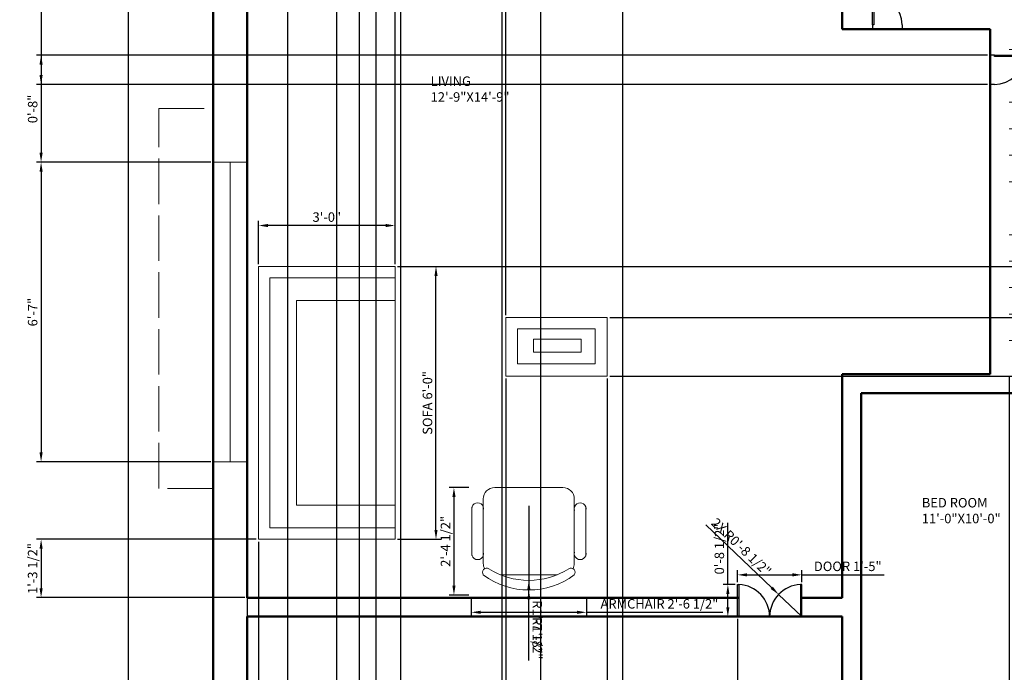
# Model space of a CAD drawing. Units: millimetres. Extents: x 3095 to 3505, y 1097 to 1734.
# Tile 2 of 5: x 3095 to 3355, y 1240 to 1412. Entities that reach past the tile are written whole.
import ezdxf

# ---------------------------------------------------------------- set-up
doc = ezdxf.new("R2010")
doc.units = ezdxf.units.MM
doc.linetypes.add('ACAD_ISO02W100', pattern=[15, 12, -3])
for name, color, linetype, lineweight, true_color in [('A-ANNO-DIMS', 32, 'Continuous', 18, 0xcd6928), ('A-AREA-IDEN', 152, 'Continuous', 18, 0x2776bb), ('A-FLOR-PATT', 241, 'Continuous', 13, 0xf7abae), ('A-FURN', 9, 'Continuous', 18, 0xafd9aa), ('A-GLAZ', 9, 'Continuous', 18, 0xd19cc7), ('A-ROOF-OVHD', 152, 'ACAD_ISO02W100', 13, 0x2776bb)]:
    doc.layers.add(name, color=color, linetype=linetype, lineweight=lineweight, true_color=true_color)
doc.layers.add('A-DOOR', color=4, linetype='Continuous', lineweight=25)
doc.layers.add('A-WALL', color=7, linetype='Continuous', lineweight=50)
doc.styles.get("Standard").update_dxf_attribs({"font": 'arial.ttf'})
doc.dimstyles.new('ISO-25', dxfattribs={"dimtxt": 2.5, "dimasz": 2.5, "dimexe": 1.25, "dimexo": 0.625, "dimtad": 1, "dimlunit": 3, "dimtxsty": 'Standard', "dimcen": 2.5, "dimadec": 0, "dimazin": 0, "dimtfac": 1, "dimtmove": 0, "dimatfit": 3, "dimfxl": 1, "dimarcsym": 0})

# ---------------------------------------------------------------- blocks, each defined once
blk = doc.blocks.new('CHAIR7')
for p, q in [((5.12, 15.04), (17.88, 15.04)), ((20, 12), (3, 12)), ((0, 9), (0, -9)), ((23, -7.44), (23, 7.44)), ((3, -12), (20, -12)), ((5.12, -15), (17.88, -15))]:
    blk.add_line(p, q)
for centre, radius, start, end in [((5.56, 13.54), 1.56, 73.7398, 286.2602), ((17.44, 13.54), 1.56, 253.7398, 106.2602), ((3, 9), 3, 90, 180), ((20, 9), 3, 62.4156, 90), ((22.34, 11.12), 1.1, 53.3099, 212.0274), ((4.82, 0), 19.64, 327.5758, 32.4242), ((7, 0), 20, 323.1301, 36.8699), ((3, -9), 3, 180, 270), ((5.56, -13.5), 1.56, 73.7398, 286.2602), ((17.44, -13.5), 1.56, 253.7398, 106.2602), ((20, -9), 3, 270, 297.5844), ((22.34, -11.12), 1.1, 147.9726, 306.6901)]:
    blk.add_arc(centre, radius, start, end)
blk = doc.blocks.new('SOFA2')
for p, q in [((-36, 0), (-36, -36)), ((36, 0), (-36, 0)), ((36, -36), (36, 0)), ((-33, -36), (-33, -3)), ((-33, -3), (33, -3)), ((33, -3), (33, -36)), ((-27, -36), (-27, -10)), ((-27, -10), (27, -10)), ((27, -10), (27, -36)), ((-36, -36), (36, -36))]:
    blk.add_line(p, q)
blk = doc.blocks.new('*U6')
for p, q in [((0, 0), (0, -6)), ((40, 0), (40, -6))]:
    blk.add_line(p, q)
blk.add_lwpolyline([(0, 0), (0, 40), (1.75, 40), (1.75, 0)], close=True)
blk.add_arc((0, 0), 40, 0, 90)
blk = doc.blocks.new('*U8')
for p, q in [((0, 0), (0, -6)), ((40, 0), (40, -6))]:
    blk.add_line(p, q)
blk.add_lwpolyline([(0, 0), (0, 40), (1.75, 40), (1.75, 0)], close=True)
blk.add_arc((0, 0), 40, 0, 90)
blk = doc.blocks.new('DR-69P')
for points in [[(1.5, 0), (0, 0), (0, 34.5), (1.5, 34.5)], [(67.5, 0), (69, 0), (69, 34.5), (67.5, 34.5)]]:
    blk.add_lwpolyline(points, close=True)
for centre, start, end in [((0, 0), 0, 87.5104), ((69, 0), 92.4896, 180)]:
    blk.add_arc(centre, 34.5, start, end)
blk = doc.blocks.new('*D11')
at = {"layer": 'A-ANNO-DIMS', "color": 0, "lineweight": -2, "transparency": 16777216}
for p, q in [((3145.24, 1677.32), (3122.17, 1677.32)), ((3123.42, 1674.82), (3123.42, 1175.82)), ((3145.24, 1173.32), (3122.17, 1173.32))]:
    blk.add_line(p, q, dxfattribs=at)
at = {"layer": 'A-ANNO-DIMS', "color": 0, "lineweight": 5, "transparency": 16777216}
for points in [[(3123, 1674.82), (3123.84, 1674.82), (3123.42, 1677.32)], [(3123, 1175.82), (3123.84, 1175.82), (3123.42, 1173.32)]]:
    blk.add_solid(points, dxfattribs=at)
at = {"layer": 'Defpoints', "color": 0, "lineweight": 5, "transparency": 16777216}
for p in [(3145.86, 1677.32), (3123.42, 1173.32), (3145.86, 1173.32)]:
    blk.add_point(p, dxfattribs=at)
at = {"layer": 'A-ANNO-DIMS', "color": 0, "transparency": 16777216, "insert": (3121.54, 1425.32), "char_height": 2.5, "attachment_point": 5, "rotation": 90}
blk.add_mtext("42'", dxfattribs=at)
blk = doc.blocks.new('*D24')
at = {"layer": 'A-ANNO-DIMS', "color": 0, "lineweight": -2, "transparency": 16777216}
for p, q in [((3213.96, 1259.39), (3213.96, 1254.21)), ((3244.38, 1259.39), (3244.38, 1254.21)), ((3216.46, 1255.46), (3241.88, 1255.46)), ((3244.38, 1255.46), (3280.34, 1255.46))]:
    blk.add_line(p, q, dxfattribs=at)
at = {"layer": 'A-ANNO-DIMS', "color": 0, "lineweight": 5, "transparency": 16777216}
for points in [[(3216.46, 1255.87), (3216.46, 1255.04), (3213.96, 1255.46)], [(3241.88, 1255.87), (3241.88, 1255.04), (3244.38, 1255.46)]]:
    blk.add_solid(points, dxfattribs=at)
at = {"layer": 'Defpoints', "color": 0, "lineweight": 5, "transparency": 16777216}
for p in [(3213.96, 1260.02), (3244.38, 1260.02), (3244.38, 1255.46)]:
    blk.add_point(p, dxfattribs=at)
at = {"layer": 'A-ANNO-DIMS', "color": 0, "transparency": 16777216, "insert": (3263.61, 1257.37), "char_height": 2.5, "attachment_point": 5}
blk.add_mtext('ARMCHAIR 2\'-6 1/2"', dxfattribs=at)
blk = doc.blocks.new('*D25')
at = {"layer": 'A-ANNO-DIMS', "color": 0, "lineweight": -2, "transparency": 16777216}
for p, q in [((3213.34, 1288.35), (3208.15, 1288.35)), ((3209.4, 1285.85), (3209.4, 1262.52)), ((3213.34, 1260.02), (3208.15, 1260.02))]:
    blk.add_line(p, q, dxfattribs=at)
at = {"layer": 'A-ANNO-DIMS', "color": 0, "lineweight": 5, "transparency": 16777216}
for points in [[(3208.98, 1285.85), (3209.82, 1285.85), (3209.4, 1288.35)], [(3208.98, 1262.52), (3209.82, 1262.52), (3209.4, 1260.02)]]:
    blk.add_solid(points, dxfattribs=at)
at = {"layer": 'Defpoints', "color": 0, "lineweight": 5, "transparency": 16777216}
for p in [(3213.96, 1288.35), (3209.4, 1260.02), (3213.96, 1260.02)]:
    blk.add_point(p, dxfattribs=at)
at = {"layer": 'A-ANNO-DIMS', "color": 0, "transparency": 16777216, "insert": (3207.48, 1274.18), "char_height": 2.5, "attachment_point": 5, "rotation": 90}
blk.add_mtext('2\'-4 1/2"', dxfattribs=at)
blk = doc.blocks.new('*D26')
at = {"layer": 'A-ANNO-DIMS', "color": 0, "lineweight": -2, "transparency": 16777216}
for p, q in [((3194.49, 1346.71), (3205.91, 1346.71)), ((3204.66, 1277.21), (3204.66, 1344.21)), ((3194.49, 1274.71), (3205.91, 1274.71))]:
    blk.add_line(p, q, dxfattribs=at)
at = {"layer": 'A-ANNO-DIMS', "color": 0, "lineweight": 5, "transparency": 16777216}
for points in [[(3204.25, 1344.21), (3205.08, 1344.21), (3204.66, 1346.71)], [(3204.25, 1277.21), (3205.08, 1277.21), (3204.66, 1274.71)]]:
    blk.add_solid(points, dxfattribs=at)
at = {"layer": 'Defpoints', "color": 0, "lineweight": 5, "transparency": 16777216}
for p in [(3193.86, 1346.71), (3204.66, 1346.71), (3193.86, 1274.71)]:
    blk.add_point(p, dxfattribs=at)
at = {"layer": 'A-ANNO-DIMS', "color": 0, "transparency": 16777216, "insert": (3202.74, 1310.71), "char_height": 2.5, "attachment_point": 5, "rotation": 90}
blk.add_mtext('SOFA 6\'-0"', dxfattribs=at)
blk = doc.blocks.new('*D27')
at = {"layer": 'A-ANNO-DIMS', "color": 0, "lineweight": -2, "transparency": 16777216}
for p, q in [((3157.86, 1347.34), (3157.86, 1358.76)), ((3193.86, 1347.34), (3193.86, 1358.76)), ((3191.36, 1357.51), (3160.36, 1357.51))]:
    blk.add_line(p, q, dxfattribs=at)
at = {"layer": 'A-ANNO-DIMS', "color": 0, "lineweight": 5, "transparency": 16777216}
for points in [[(3160.36, 1357.93), (3160.36, 1357.09), (3157.86, 1357.51)], [(3191.36, 1357.93), (3191.36, 1357.09), (3193.86, 1357.51)]]:
    blk.add_solid(points, dxfattribs=at)
at = {"layer": 'Defpoints', "color": 0, "lineweight": 5, "transparency": 16777216}
for p in [(3157.86, 1357.51), (3157.86, 1346.71), (3193.86, 1346.71)]:
    blk.add_point(p, dxfattribs=at)
at = {"layer": 'A-ANNO-DIMS', "color": 0, "transparency": 16777216, "insert": (3175.86, 1359.41), "char_height": 2.5, "attachment_point": 5}
blk.add_mtext('3\'-0"', dxfattribs=at)
blk = doc.blocks.new('*D28')
at = {"layer": 'A-ANNO-DIMS', "color": 0, "lineweight": -2, "transparency": 16777216}
for p, q in [((3284.21, 1263.42), (3284.21, 1266.59)), ((3286.71, 1265.34), (3298.68, 1265.34)), ((3301.18, 1263.42), (3301.18, 1266.59)), ((3301.18, 1265.34), (3322.9, 1265.34))]:
    blk.add_line(p, q, dxfattribs=at)
at = {"layer": 'A-ANNO-DIMS', "color": 0, "lineweight": 5, "transparency": 16777216}
for points in [[(3286.71, 1265.76), (3286.71, 1264.92), (3284.21, 1265.34)], [(3298.68, 1265.76), (3298.68, 1264.92), (3301.18, 1265.34)]]:
    blk.add_solid(points, dxfattribs=at)
at = {"layer": 'Defpoints', "color": 0, "lineweight": 5, "transparency": 16777216}
for p in [(3301.18, 1265.34), (3284.21, 1262.8), (3301.18, 1262.8)]:
    blk.add_point(p, dxfattribs=at)
at = {"layer": 'A-ANNO-DIMS', "color": 0, "transparency": 16777216, "insert": (3313.29, 1267.26), "char_height": 2.5, "attachment_point": 5}
blk.add_mtext('DOOR 1\'-5"', dxfattribs=at)
blk = doc.blocks.new('*D29')
at = {"layer": 'A-ANNO-DIMS', "color": 0, "lineweight": -2, "transparency": 16777216}
for p, q in [((3281.66, 1262.8), (3281.66, 1279.02)), ((3283.58, 1262.8), (3280.41, 1262.8)), ((3281.66, 1256.81), (3281.66, 1260.3)), ((3283.58, 1254.31), (3280.41, 1254.31))]:
    blk.add_line(p, q, dxfattribs=at)
at = {"layer": 'A-ANNO-DIMS', "color": 0, "lineweight": 5, "transparency": 16777216}
for points in [[(3281.24, 1260.3), (3282.08, 1260.3), (3281.66, 1262.8)], [(3281.24, 1256.81), (3282.08, 1256.81), (3281.66, 1254.31)]]:
    blk.add_solid(points, dxfattribs=at)
at = {"layer": 'Defpoints', "color": 0, "lineweight": 5, "transparency": 16777216}
for p in [(3281.66, 1262.8), (3284.21, 1262.8), (3284.21, 1254.31)]:
    blk.add_point(p, dxfattribs=at)
at = {"layer": 'A-ANNO-DIMS', "color": 0, "transparency": 16777216, "insert": (3279.74, 1272.16), "char_height": 2.5, "attachment_point": 5, "rotation": 90}
blk.add_mtext('0\'-8 1/2"', dxfattribs=at)
blk = doc.blocks.new('*D36')
at = {"layer": 'A-ANNO-DIMS', "color": 0, "lineweight": -2, "transparency": 16777216}
for p, q in [((3145.24, 1477.6), (3099.22, 1477.6)), ((3100.47, 1475.1), (3100.47, 1376.7)), ((3145.24, 1374.2), (3099.22, 1374.2))]:
    blk.add_line(p, q, dxfattribs=at)
at = {"layer": 'A-ANNO-DIMS', "color": 0, "lineweight": 5, "transparency": 16777216}
for points in [[(3100.06, 1475.1), (3100.89, 1475.1), (3100.47, 1477.6)], [(3100.06, 1376.7), (3100.89, 1376.7), (3100.47, 1374.2)]]:
    blk.add_solid(points, dxfattribs=at)
at = {"layer": 'Defpoints', "color": 0, "lineweight": 5, "transparency": 16777216}
for p in [(3145.86, 1477.6), (3100.47, 1374.2), (3145.86, 1374.2)]:
    blk.add_point(p, dxfattribs=at)
at = {"layer": 'A-ANNO-DIMS', "color": 0, "transparency": 16777216, "insert": (3098.56, 1425.9), "char_height": 2.5, "attachment_point": 5, "rotation": 90}
blk.add_mtext('8\'-7 1/2"', dxfattribs=at)
blk = doc.blocks.new('*D37')
at = {"layer": 'A-ANNO-DIMS', "color": 0, "lineweight": -2, "transparency": 16777216}
for p, q in [((3145.24, 1374.2), (3099.22, 1374.2)), ((3100.47, 1371.7), (3100.47, 1297.63)), ((3145.24, 1295.13), (3099.22, 1295.13))]:
    blk.add_line(p, q, dxfattribs=at)
at = {"layer": 'A-ANNO-DIMS', "color": 0, "lineweight": 5, "transparency": 16777216}
for points in [[(3100.06, 1371.7), (3100.89, 1371.7), (3100.47, 1374.2)], [(3100.06, 1297.63), (3100.89, 1297.63), (3100.47, 1295.13)]]:
    blk.add_solid(points, dxfattribs=at)
at = {"layer": 'Defpoints', "color": 0, "lineweight": 5, "transparency": 16777216}
for p in [(3145.86, 1374.2), (3100.47, 1295.13), (3145.86, 1295.13)]:
    blk.add_point(p, dxfattribs=at)
at = {"layer": 'A-ANNO-DIMS', "color": 0, "transparency": 16777216, "insert": (3098.57, 1334.66), "char_height": 2.5, "attachment_point": 5, "rotation": 90}
blk.add_mtext('6\'-7"', dxfattribs=at)
blk = doc.blocks.new('*D49')
at = {"layer": 'A-ANNO-DIMS', "color": 0, "lineweight": -2, "transparency": 16777216}
for p, q in [((3154.86, 1588.17), (3154.86, 1134.75)), ((3188.81, 1588.17), (3188.81, 1134.75)), ((3157.36, 1136), (3186.31, 1136))]:
    blk.add_line(p, q, dxfattribs=at)
at = {"layer": 'A-ANNO-DIMS', "color": 0, "lineweight": 5, "transparency": 16777216}
for points in [[(3157.36, 1136.41), (3157.36, 1135.58), (3154.86, 1136)], [(3186.31, 1136.41), (3186.31, 1135.58), (3188.81, 1136)]]:
    blk.add_solid(points, dxfattribs=at)
at = {"layer": 'Defpoints', "color": 0, "lineweight": 5, "transparency": 16777216}
for p in [(3154.86, 1588.8), (3188.81, 1588.8), (3188.81, 1136)]:
    blk.add_point(p, dxfattribs=at)
at = {"layer": 'A-ANNO-DIMS', "color": 0, "transparency": 16777216, "insert": (3171.84, 1137.9), "char_height": 2.5, "attachment_point": 5}
blk.add_mtext('2\'-10"', dxfattribs=at)
blk = doc.blocks.new('*D50')
at = {"layer": 'A-ANNO-DIMS', "color": 0, "lineweight": -2, "transparency": 16777216}
for p, q in [((3222, 1588.17), (3222, 1134.75)), ((3253.86, 1588.17), (3253.86, 1134.75)), ((3224.5, 1136), (3251.36, 1136))]:
    blk.add_line(p, q, dxfattribs=at)
at = {"layer": 'A-ANNO-DIMS', "color": 0, "lineweight": 5, "transparency": 16777216}
for points in [[(3224.5, 1136.41), (3224.5, 1135.58), (3222, 1136)], [(3251.36, 1136.41), (3251.36, 1135.58), (3253.86, 1136)]]:
    blk.add_solid(points, dxfattribs=at)
at = {"layer": 'Defpoints', "color": 0, "lineweight": 5, "transparency": 16777216}
for p in [(3222, 1588.8), (3253.86, 1588.8), (3253.86, 1136)]:
    blk.add_point(p, dxfattribs=at)
at = {"layer": 'A-ANNO-DIMS', "color": 0, "transparency": 16777216, "insert": (3237.93, 1137.9), "char_height": 2.5, "attachment_point": 5}
blk.add_mtext('2\'-8"', dxfattribs=at)
blk = doc.blocks.new('*D52')
at = {"layer": 'A-ANNO-DIMS', "color": 0, "lineweight": -2, "transparency": 16777216}
for p, q in [((3178.42, 1456.63), (3178.42, 1134.75)), ((3232.26, 1456.63), (3232.26, 1134.75)), ((3180.92, 1136), (3229.76, 1136))]:
    blk.add_line(p, q, dxfattribs=at)
at = {"layer": 'A-ANNO-DIMS', "color": 0, "lineweight": 5, "transparency": 16777216}
for points in [[(3180.92, 1136.41), (3180.92, 1135.58), (3178.42, 1136)], [(3229.76, 1136.41), (3229.76, 1135.58), (3232.26, 1136)]]:
    blk.add_solid(points, dxfattribs=at)
at = {"layer": 'Defpoints', "color": 0, "lineweight": 5, "transparency": 16777216}
for p in [(3178.42, 1457.25), (3232.26, 1457.25), (3232.26, 1136)]:
    blk.add_point(p, dxfattribs=at)
at = {"layer": 'A-ANNO-DIMS', "color": 0, "transparency": 16777216, "insert": (3205.34, 1137.9), "char_height": 2.5, "attachment_point": 5}
blk.add_mtext('4\'-6"', dxfattribs=at)
blk = doc.blocks.new('*D57')
at = {"layer": 'A-ANNO-DIMS', "color": 0, "lineweight": -2, "transparency": 16777216}
for p, q in [((3165.47, 1598.31), (3165.47, 1134.75)), ((3184.42, 1598.31), (3184.42, 1134.75)), ((3167.97, 1136), (3181.92, 1136))]:
    blk.add_line(p, q, dxfattribs=at)
at = {"layer": 'A-ANNO-DIMS', "color": 0, "lineweight": 5, "transparency": 16777216}
for points in [[(3167.97, 1136.41), (3167.97, 1135.58), (3165.47, 1136)], [(3181.92, 1136.41), (3181.92, 1135.58), (3184.42, 1136)]]:
    blk.add_solid(points, dxfattribs=at)
at = {"layer": 'Defpoints', "color": 0, "lineweight": 5, "transparency": 16777216}
for p in [(3165.47, 1598.93), (3184.42, 1598.93), (3184.42, 1136)]:
    blk.add_point(p, dxfattribs=at)
at = {"layer": 'A-ANNO-DIMS', "color": 0, "transparency": 16777216, "insert": (3174.95, 1137.88), "char_height": 2.5, "attachment_point": 5}
blk.add_mtext('1\'-7"', dxfattribs=at)
blk = doc.blocks.new('*D62')
at = {"layer": 'A-ANNO-DIMS', "color": 0, "lineweight": -2, "transparency": 16777216}
for p, q in [((3350.19, 1402.48), (3099.22, 1402.48)), ((3100.47, 1399.98), (3100.47, 1397.22)), ((3350.19, 1394.72), (3099.22, 1394.72)), ((3100.47, 1394.72), (3100.47, 1384.32))]:
    blk.add_line(p, q, dxfattribs=at)
at = {"layer": 'A-ANNO-DIMS', "color": 0, "lineweight": 5, "transparency": 16777216}
for points in [[(3100.06, 1399.98), (3100.89, 1399.98), (3100.47, 1402.48)], [(3100.06, 1397.22), (3100.89, 1397.22), (3100.47, 1394.72)]]:
    blk.add_solid(points, dxfattribs=at)
at = {"layer": 'Defpoints', "color": 0, "lineweight": 5, "transparency": 16777216}
for p in [(3350.82, 1402.48), (3100.47, 1394.72), (3350.82, 1394.72)]:
    blk.add_point(p, dxfattribs=at)
at = {"layer": 'A-ANNO-DIMS', "color": 0, "transparency": 16777216, "insert": (3098.57, 1388.27), "char_height": 2.5, "attachment_point": 5, "rotation": 90}
blk.add_mtext('0\'-8"', dxfattribs=at)
blk = doc.blocks.new('*D64')
at = {"layer": 'A-ANNO-DIMS', "color": 0, "lineweight": -2, "transparency": 16777216}
for p, q in [((3355.86, 1317.69), (3355.86, 1134.75)), ((3356.76, 1312.81), (3356.76, 1134.75)), ((3353.36, 1136), (3342.97, 1136)), ((3356.76, 1136), (3355.86, 1136)), ((3359.26, 1136), (3361.76, 1136))]:
    blk.add_line(p, q, dxfattribs=at)
at = {"layer": 'A-ANNO-DIMS', "color": 0, "lineweight": 5, "transparency": 16777216}
for points in [[(3353.36, 1136.41), (3353.36, 1135.58), (3355.86, 1136)], [(3359.26, 1136.41), (3359.26, 1135.58), (3356.76, 1136)]]:
    blk.add_solid(points, dxfattribs=at)
at = {"layer": 'Defpoints', "color": 0, "lineweight": 5, "transparency": 16777216}
for p in [(3355.86, 1318.32), (3356.76, 1313.43), (3355.86, 1136)]:
    blk.add_point(p, dxfattribs=at)
at = {"layer": 'A-ANNO-DIMS', "color": 0, "transparency": 16777216, "insert": (3346.91, 1137.9), "char_height": 2.5, "attachment_point": 5}
blk.add_mtext('0\'-1"', dxfattribs=at)
blk = doc.blocks.new('*D65')
at = {"layer": 'A-ANNO-DIMS', "color": 0, "lineweight": -2, "transparency": 16777216}
for p, q in [((3178.42, 1456.63), (3178.42, 1134.75)), ((3154.86, 1439.69), (3154.86, 1134.75)), ((3175.92, 1136), (3157.36, 1136))]:
    blk.add_line(p, q, dxfattribs=at)
at = {"layer": 'A-ANNO-DIMS', "color": 0, "lineweight": 5, "transparency": 16777216}
for points in [[(3157.36, 1136.41), (3157.36, 1135.58), (3154.86, 1136)], [(3175.92, 1136.41), (3175.92, 1135.58), (3178.42, 1136)]]:
    blk.add_solid(points, dxfattribs=at)
at = {"layer": 'Defpoints', "color": 0, "lineweight": 5, "transparency": 16777216}
for p in [(3178.42, 1457.25), (3154.86, 1440.32), (3154.86, 1136)]:
    blk.add_point(p, dxfattribs=at)
at = {"layer": 'A-ANNO-DIMS', "color": 0, "transparency": 16777216, "insert": (3166.64, 1137.91), "char_height": 2.5, "attachment_point": 5}
blk.add_mtext('1\'-11 1/2"', dxfattribs=at)
blk = doc.blocks.new('*D67')
at = {"layer": 'A-ANNO-DIMS', "color": 0, "lineweight": -2, "transparency": 16777216}
for p, q in [((3154.86, 1253.69), (3154.86, 1134.75)), ((3284.21, 1253.69), (3284.21, 1134.75)), ((3281.71, 1136), (3157.36, 1136))]:
    blk.add_line(p, q, dxfattribs=at)
at = {"layer": 'A-ANNO-DIMS', "color": 0, "lineweight": 5, "transparency": 16777216}
for points in [[(3157.36, 1136.41), (3157.36, 1135.58), (3154.86, 1136)], [(3281.71, 1136.41), (3281.71, 1135.58), (3284.21, 1136)]]:
    blk.add_solid(points, dxfattribs=at)
at = {"layer": 'Defpoints', "color": 0, "lineweight": 5, "transparency": 16777216}
for p in [(3154.86, 1254.32), (3284.21, 1254.31), (3154.86, 1136)]:
    blk.add_point(p, dxfattribs=at)
at = {"layer": 'A-ANNO-DIMS', "color": 0, "transparency": 16777216, "insert": (3219.53, 1137.91), "char_height": 2.5, "attachment_point": 5}
blk.add_mtext('10\'-9 1/2"', dxfattribs=at)
blk = doc.blocks.new('*D68')
at = {"layer": 'A-ANNO-DIMS', "color": 0, "lineweight": -2, "transparency": 16777216}
for p, q in [((3223.06, 1317.18), (3223.06, 1134.75)), ((3249.85, 1317.18), (3249.85, 1134.75)), ((3225.56, 1136), (3247.35, 1136))]:
    blk.add_line(p, q, dxfattribs=at)
at = {"layer": 'A-ANNO-DIMS', "color": 0, "lineweight": 5, "transparency": 16777216}
for points in [[(3225.56, 1136.41), (3225.56, 1135.58), (3223.06, 1136)], [(3247.35, 1136.41), (3247.35, 1135.58), (3249.85, 1136)]]:
    blk.add_solid(points, dxfattribs=at)
at = {"layer": 'Defpoints', "color": 0, "lineweight": 5, "transparency": 16777216}
for p in [(3223.06, 1317.8), (3249.85, 1317.8), (3249.85, 1136)]:
    blk.add_point(p, dxfattribs=at)
at = {"layer": 'A-ANNO-DIMS', "color": 0, "transparency": 16777216, "insert": (3236.46, 1137.9), "char_height": 2.5, "attachment_point": 5}
blk.add_mtext('2\'-3"', dxfattribs=at)
blk = doc.blocks.new('*D69')
at = {"layer": 'A-ANNO-DIMS', "color": 0, "lineweight": -2, "transparency": 16777216}
for p, q in [((3250.48, 1333.27), (3504.29, 1333.27)), ((3503.04, 1330.77), (3503.04, 1320.3)), ((3250.48, 1317.8), (3504.29, 1317.8))]:
    blk.add_line(p, q, dxfattribs=at)
at = {"layer": 'A-ANNO-DIMS', "color": 0, "lineweight": 5, "transparency": 16777216}
for points in [[(3502.63, 1330.77), (3503.46, 1330.77), (3503.04, 1333.27)], [(3502.63, 1320.3), (3503.46, 1320.3), (3503.04, 1317.8)]]:
    blk.add_solid(points, dxfattribs=at)
at = {"layer": 'Defpoints', "color": 0, "lineweight": 5, "transparency": 16777216}
for p in [(3249.85, 1333.27), (3249.85, 1317.8), (3503.04, 1317.8)]:
    blk.add_point(p, dxfattribs=at)
at = {"layer": 'A-ANNO-DIMS', "color": 0, "transparency": 16777216, "insert": (3501.12, 1325.54), "char_height": 2.5, "attachment_point": 5, "rotation": 90}
blk.add_mtext('1\'-3 1/2"', dxfattribs=at)
blk = doc.blocks.new('*D70')
at = {"layer": 'A-ANNO-DIMS', "color": 0, "lineweight": -2, "transparency": 16777216}
for p, q in [((3165.47, 1598.31), (3165.47, 1134.75)), ((3154.86, 1588.17), (3154.86, 1134.75)), ((3157.36, 1136), (3162.97, 1136)), ((3165.47, 1136), (3183.64, 1136))]:
    blk.add_line(p, q, dxfattribs=at)
at = {"layer": 'A-ANNO-DIMS', "color": 0, "lineweight": 5, "transparency": 16777216}
for points in [[(3157.36, 1136.41), (3157.36, 1135.58), (3154.86, 1136)], [(3162.97, 1136.41), (3162.97, 1135.58), (3165.47, 1136)]]:
    blk.add_solid(points, dxfattribs=at)
at = {"layer": 'Defpoints', "color": 0, "lineweight": 5, "transparency": 16777216}
for p in [(3165.47, 1598.93), (3154.86, 1588.8), (3165.47, 1136)]:
    blk.add_point(p, dxfattribs=at)
at = {"layer": 'A-ANNO-DIMS', "color": 0, "transparency": 16777216, "insert": (3175.81, 1137.91), "char_height": 2.5, "attachment_point": 5}
blk.add_mtext('0\'-10 1/2"', dxfattribs=at)
blk = doc.blocks.new('*D72')
at = {"layer": 'A-ANNO-DIMS', "color": 0, "lineweight": -2, "transparency": 16777216}
for p, q in [((3195.33, 1651.97), (3195.33, 1134.75)), ((3188.81, 1649.1), (3188.81, 1134.75)), ((3188.81, 1136), (3172.59, 1136)), ((3192.83, 1136), (3191.31, 1136))]:
    blk.add_line(p, q, dxfattribs=at)
at = {"layer": 'A-ANNO-DIMS', "color": 0, "lineweight": 5, "transparency": 16777216}
for points in [[(3191.31, 1136.41), (3191.31, 1135.58), (3188.81, 1136)], [(3192.83, 1136.41), (3192.83, 1135.58), (3195.33, 1136)]]:
    blk.add_solid(points, dxfattribs=at)
at = {"layer": 'Defpoints', "color": 0, "lineweight": 5, "transparency": 16777216}
for p in [(3195.33, 1652.6), (3188.81, 1649.73), (3188.81, 1136)]:
    blk.add_point(p, dxfattribs=at)
at = {"layer": 'A-ANNO-DIMS', "color": 0, "transparency": 16777216, "insert": (3179.45, 1137.91), "char_height": 2.5, "attachment_point": 5}
blk.add_mtext('0\'-6 1/2"', dxfattribs=at)
blk = doc.blocks.new('*D74')
at = {"layer": 'A-ANNO-DIMS', "color": 0, "lineweight": -2, "transparency": 16777216}
for p, q in [((3157.86, 1274.09), (3157.86, 1134.75)), ((3154.86, 1258.69), (3154.86, 1134.75)), ((3152.36, 1136), (3141.97, 1136)), ((3157.86, 1136), (3154.86, 1136)), ((3160.36, 1136), (3162.86, 1136))]:
    blk.add_line(p, q, dxfattribs=at)
at = {"layer": 'A-ANNO-DIMS', "color": 0, "lineweight": 5, "transparency": 16777216}
for points in [[(3152.36, 1136.41), (3152.36, 1135.58), (3154.86, 1136)], [(3160.36, 1136.41), (3160.36, 1135.58), (3157.86, 1136)]]:
    blk.add_solid(points, dxfattribs=at)
at = {"layer": 'Defpoints', "color": 0, "lineweight": 5, "transparency": 16777216}
for p in [(3157.86, 1274.71), (3154.86, 1259.32), (3154.86, 1136)]:
    blk.add_point(p, dxfattribs=at)
at = {"layer": 'A-ANNO-DIMS', "color": 0, "transparency": 16777216, "insert": (3145.91, 1137.9), "char_height": 2.5, "attachment_point": 5}
blk.add_mtext('0\'-3"', dxfattribs=at)
blk = doc.blocks.new('*D75')
at = {"layer": 'A-ANNO-DIMS', "color": 0, "lineweight": -2, "transparency": 16777216}
for p, q in [((3157.24, 1274.71), (3099.22, 1274.71)), ((3100.47, 1272.21), (3100.47, 1261.82)), ((3154.24, 1259.32), (3099.22, 1259.32))]:
    blk.add_line(p, q, dxfattribs=at)
at = {"layer": 'A-ANNO-DIMS', "color": 0, "lineweight": 5, "transparency": 16777216}
for points in [[(3100.06, 1272.21), (3100.89, 1272.21), (3100.47, 1274.71)], [(3100.06, 1261.82), (3100.89, 1261.82), (3100.47, 1259.32)]]:
    blk.add_solid(points, dxfattribs=at)
at = {"layer": 'Defpoints', "color": 0, "lineweight": 5, "transparency": 16777216}
for p in [(3157.86, 1274.71), (3100.47, 1259.32), (3154.86, 1259.32)]:
    blk.add_point(p, dxfattribs=at)
at = {"layer": 'A-ANNO-DIMS', "color": 0, "transparency": 16777216, "insert": (3098.56, 1267.01), "char_height": 2.5, "attachment_point": 5, "rotation": 90}
blk.add_mtext('1\'-3 1/2"', dxfattribs=at)
blk = doc.blocks.new('*D76')
at = {"layer": 'A-ANNO-DIMS', "color": 0, "lineweight": -2, "transparency": 16777216}
for p, q in [((3193.86, 1347.34), (3193.86, 1729.27)), ((3196.36, 1728.02), (3220.56, 1728.02)), ((3223.06, 1333.89), (3223.06, 1729.27))]:
    blk.add_line(p, q, dxfattribs=at)
at = {"layer": 'A-ANNO-DIMS', "color": 0, "lineweight": 5, "transparency": 16777216}
for points in [[(3196.36, 1728.43), (3196.36, 1727.6), (3193.86, 1728.02)], [(3220.56, 1728.43), (3220.56, 1727.6), (3223.06, 1728.02)]]:
    blk.add_solid(points, dxfattribs=at)
at = {"layer": 'Defpoints', "color": 0, "lineweight": 5, "transparency": 16777216}
for p in [(3223.06, 1728.02), (3193.86, 1346.71), (3223.06, 1333.27)]:
    blk.add_point(p, dxfattribs=at)
at = {"layer": 'A-ANNO-DIMS', "color": 0, "transparency": 16777216, "insert": (3208.46, 1729.92), "char_height": 2.5, "attachment_point": 5}
blk.add_mtext('2\'-5"', dxfattribs=at)
blk = doc.blocks.new('*D77')
at = {"layer": 'A-ANNO-DIMS', "color": 0, "lineweight": -2, "transparency": 16777216}
for p, q in [((3194.49, 1346.71), (3504.29, 1346.71)), ((3503.04, 1344.21), (3503.04, 1320.3)), ((3250.48, 1317.8), (3504.29, 1317.8))]:
    blk.add_line(p, q, dxfattribs=at)
at = {"layer": 'A-ANNO-DIMS', "color": 0, "lineweight": 5, "transparency": 16777216}
for points in [[(3502.63, 1344.21), (3503.46, 1344.21), (3503.04, 1346.71)], [(3502.63, 1320.3), (3503.46, 1320.3), (3503.04, 1317.8)]]:
    blk.add_solid(points, dxfattribs=at)
at = {"layer": 'Defpoints', "color": 0, "lineweight": 5, "transparency": 16777216}
for p in [(3193.86, 1346.71), (3249.85, 1317.8), (3503.04, 1317.8)]:
    blk.add_point(p, dxfattribs=at)
at = {"layer": 'A-ANNO-DIMS', "color": 0, "transparency": 16777216, "insert": (3501.14, 1332.26), "char_height": 2.5, "attachment_point": 5, "rotation": 90}
blk.add_mtext('2\'-5"', dxfattribs=at)
blk = doc.blocks.new('*D91')
at = {"layer": 'A-ANNO-DIMS', "color": 0, "lineweight": -2, "transparency": 16777216}
for p, q in [((3229.15, 1281.35), (3229.15, 1261.35)), ((3229.15, 1244.21), (3229.15, 1258.85))]:
    blk.add_line(p, q, dxfattribs=at)
at = {"layer": 'A-ANNO-DIMS', "color": 0, "lineweight": 5, "transparency": 16777216}
blk.add_solid([(3229.57, 1258.85), (3228.73, 1258.85), (3229.15, 1261.35)], dxfattribs=at)
at = {"layer": 'Defpoints', "color": 0, "lineweight": 5, "transparency": 16777216}
for p in [(3229.15, 1281.35), (3229.15, 1261.35)]:
    blk.add_point(p, dxfattribs=at)
at = {"layer": 'A-ANNO-DIMS', "color": 0, "transparency": 16777216, "insert": (3231.05, 1249.35), "char_height": 2.5, "attachment_point": 5, "rotation": 270.001}
blk.add_mtext('R1\'-8"', dxfattribs=at)
blk = doc.blocks.new('*D92')
at = {"layer": 'A-ANNO-DIMS', "color": 0, "lineweight": -2, "transparency": 16777216}
for p, q in [((3229.15, 1283.53), (3229.15, 1263.89)), ((3229.15, 1242.77), (3229.15, 1261.39))]:
    blk.add_line(p, q, dxfattribs=at)
at = {"layer": 'A-ANNO-DIMS', "color": 0, "lineweight": 5, "transparency": 16777216}
blk.add_solid([(3229.57, 1261.39), (3228.73, 1261.39), (3229.15, 1263.89)], dxfattribs=at)
at = {"layer": 'Defpoints', "color": 0, "lineweight": 5, "transparency": 16777216}
for p in [(3229.15, 1283.53), (3229.15, 1263.89)]:
    blk.add_point(p, dxfattribs=at)
at = {"layer": 'A-ANNO-DIMS', "color": 0, "transparency": 16777216, "insert": (3231.07, 1250.83), "char_height": 2.5, "attachment_point": 5, "rotation": 270.001}
blk.add_mtext('R1\'-7 1/2"', dxfattribs=at)
blk = doc.blocks.new('*D93')
at = {"layer": 'A-ANNO-DIMS', "color": 0, "lineweight": -2, "transparency": 16777216}
for p, q in [((3275.89, 1278.52), (3293.24, 1261.91)), ((3301.18, 1254.31), (3295.05, 1260.18))]:
    blk.add_line(p, q, dxfattribs=at)
at = {"layer": 'A-ANNO-DIMS', "color": 0, "lineweight": 5, "transparency": 16777216}
blk.add_solid([(3293.53, 1262.21), (3292.95, 1261.61), (3295.05, 1260.18)], dxfattribs=at)
at = {"layer": 'Defpoints', "color": 0, "lineweight": 5, "transparency": 16777216}
for p in [(3295.05, 1260.18), (3301.18, 1254.31)]:
    blk.add_point(p, dxfattribs=at)
at = {"layer": 'A-ANNO-DIMS', "color": 0, "transparency": 16777216, "insert": (3284.99, 1272.47), "char_height": 2.5, "attachment_point": 5, "rotation": 316.2442}
blk.add_mtext('2X R0\'-8 1/2"', dxfattribs=at)

msp = doc.modelspace()

# ---------------------------------------------------------------- hatches: boundary and pattern name
at = {"layer": 'A-FLOR-PATT'}
h = msp.add_hatch(dxfattribs=at)
h.set_pattern_fill('ANGLE', color=256)
h.set_pattern_definition([(0, (0, 0), (0, 6.985), [5.08, -1.905]), (90, (0, 0), (-6.985, 4e-16), [5.08, -1.905])])
h.paths.add_polyline_path([(3311.862, 1668.316), (3273.923, 1668.316), (3273.923, 1664.496), (3270.819, 1664.496), (3271.774, 1661.631, -0.5301431), (3268.909, 1652.448, -0.530136), (3266.044, 1661.631), (3266.999, 1664.496), (3265.566, 1664.496), (3265.566, 1663.78), (3264.134, 1663.78), (3264.134, 1664.496), (3263.895, 1664.496), (3263.895, 1668.316), (3258.862, 1668.316), (3258.862, 1527.316), (3311.862, 1527.316), (3311.862, 1534.492), (3307.983, 1534.492), (3307.983, 1534.831), (3307.991, 1534.831, -0.2562565), (3311.862, 1541.211)])
h.paths.add_polyline_path([(3448.862, 1409.316), (3355.862, 1409.316), (3355.862, 1402.478), (3359.742, 1402.478), (3359.742, 1402.139), (3359.734, 1402.139, -0.2562565), (3355.862, 1395.759), (3355.862, 1366.316), (3424.964, 1366.316), (3424.964, 1370.136), (3428.068, 1370.136), (3427.113, 1373.001, -0.4652664), (3428.865, 1381.717, -0.3212229), (3431.09, 1381.717, -0.4652592), (3432.843, 1373.001), (3431.888, 1370.136), (3433.32, 1370.136), (3433.32, 1370.853), (3434.753, 1370.853), (3434.992, 1370.136), (3434.992, 1366.316), (3448.862, 1366.316)])
h.paths.add_polyline_path([(3428.308, 1345.964, -0.4652592), (3426.555, 1354.679), (3427.51, 1357.544), (3426.078, 1357.544), (3426.078, 1356.828), (3424.645, 1356.828), (3424.407, 1357.544), (3424.407, 1361.316), (3355.862, 1361.316), (3355.862, 1322.305, -0.0398063), (3357.095, 1322.349), (3357.095, 1322.357), (3356.756, 1322.357, -0.2743513), (3363.565, 1318.316), (3448.862, 1318.316), (3448.862, 1361.316), (3434.434, 1361.316), (3434.434, 1357.544), (3431.331, 1357.544), (3432.286, 1354.679, -0.4652664), (3430.533, 1345.964, -0.3212229)])

# ---------------------------------------------------------------- linework, layer by layer
at = {"layer": 'A-FURN'}
for points in [[(3223.059, 1333.27), (3249.851, 1333.27), (3249.851, 1317.802), (3223.059, 1317.802)], [(3226.142, 1330.207), (3246.629, 1330.207), (3246.629, 1321.025), (3226.142, 1321.025)], [(3230.354, 1327.529), (3242.991, 1327.529), (3242.991, 1324.086), (3230.354, 1324.086)]]:
    msp.add_lwpolyline(points, close=True, dxfattribs=at)
at = {"layer": 'A-GLAZ'}
for p, q in [((3145.862, 1374.196), (3154.862, 1374.196)), ((3145.862, 1295.134), (3145.862, 1374.196)), ((3145.862, 1374.196), (3150.362, 1374.196)), ((3150.362, 1374.196), (3150.362, 1295.134)), ((3154.862, 1374.196), (3154.862, 1295.134)), ((3154.862, 1295.134), (3145.862, 1295.134))]:
    msp.add_line(p, q, dxfattribs=at)
at = {"layer": 'A-ROOF-OVHD'}
for p, q in [((3131.524, 1288.161), (3131.524, 1388.41)), ((3131.524, 1388.41), (3145.862, 1388.41)), ((3145.862, 1288.161), (3131.524, 1288.161))]:
    msp.add_line(p, q, dxfattribs=at)
at = {"layer": 'A-WALL'}
for p, q in [((3145.862, 1173.316), (3145.862, 1677.316)), ((3311.862, 1522.316), (3311.862, 1409.316)), ((3154.862, 1259.316), (3154.862, 1435.316)), ((3311.862, 1409.316), (3350.862, 1409.316)), ((3350.862, 1409.316), (3350.862, 1318.316)), ((3311.862, 1318.316), (3350.862, 1318.316)), ((3311.862, 1318.316), (3311.862, 1259.316)), ((3316.862, 1313.316), (3448.862, 1313.316)), ((3316.862, 1313.316), (3316.862, 1182.316)), ((3284.575, 1259.316), (3154.862, 1259.316)), ((3311.862, 1259.316), (3300.807, 1259.316)), ((3154.862, 1182.316), (3154.862, 1254.316)), ((3311.862, 1254.316), (3154.862, 1254.316)), ((3311.862, 1254.316), (3311.862, 1182.316))]:
    msp.add_line(p, q, dxfattribs=at)

# ---------------------------------------------------------------- block references
at = {"layer": 'A-DOOR'}
for name, p, xscale, yscale, zscale in [('*U6', (3319.865, 1410.463), 0.1939559161486229, 0.1939559161486229, 0.1939559161486229), ('DR-69P', (3284.206, 1254.31), 0.2459480974031906, 0.2459480974031906, 0.2459480974031906)]:
    msp.add_blockref(name, p, dxfattribs=dict(at, xscale=xscale, yscale=yscale, zscale=zscale))
at = {"layer": 'A-DOOR', "xscale": 0.1939559161486229, "yscale": 0.1939559161486229, "zscale": 0.1939559161486229, "rotation": 270}
msp.add_blockref('*U8', (3351.983, 1402.478), dxfattribs=at)
at = {"layer": 'A-FURN'}
for name, p, rotation in [('SOFA2', (3157.862, 1310.711), 90), ('CHAIR7', (3229.149, 1288.351), 270)]:
    msp.add_blockref(name, p, dxfattribs=dict(at, rotation=rotation))

# ---------------------------------------------------------------- texts
at = {"layer": 'A-AREA-IDEN', "char_height": 2.5, "attachment_point": 1}
for s, width, insert in [('LIVING\\P12\'-9"X14\'-9"', 93.21131, (3203.251, 1396.84)), ('BED ROOM\\P11\'-0"X10\'-0"', 108.17348, (3332.835, 1285.62))]:
    msp.add_mtext_dynamic_manual_height_columns(s, width=width, gutter_width=12.5, heights=[0], dxfattribs=dict(at, insert=insert))

# ---------------------------------------------------------------- dimensions: what is measured, and where the dimension line sits
at = {"layer": 'A-ANNO-DIMS'}
for base, p1, p2, picture, middle in [((3223.059, 1728.017), (3193.862, 1346.711), (3223.059, 1333.27), '*D76', (3208.461, 1729.919)), ((3188.808, 1135.996), (3195.33, 1652.599), (3188.808, 1649.727), '*D72', (3179.447, 1137.914)), ((3165.474, 1135.996), (3154.862, 1588.796), (3165.474, 1598.93), '*D70', (3175.806, 1137.914)), ((3184.422, 1135.996), (3165.474, 1598.93), (3184.422, 1598.93), '*D57', (3174.948, 1137.877)), ((3188.808, 1135.996), (3154.862, 1588.796), (3188.808, 1588.796), '*D49', (3171.835, 1137.898)), ((3253.862, 1135.996), (3221.995, 1588.796), (3253.862, 1588.796), '*D50', (3237.929, 1137.898)), ((3154.862, 1135.996), (3178.42, 1457.251), (3154.862, 1440.316), '*D65', (3166.641, 1137.914)), ((3232.262, 1135.996), (3178.42, 1457.251), (3232.262, 1457.251), '*D52', (3205.341, 1137.898)), ((3249.851, 1135.996), (3223.059, 1317.802), (3249.851, 1317.802), '*D68', (3236.455, 1137.899)), ((3355.862, 1135.996), (3356.756, 1313.435), (3355.862, 1318.316), '*D64', (3346.915, 1137.898)), ((3154.862, 1135.996), (3157.862, 1274.711), (3154.862, 1259.316), '*D74', (3145.915, 1137.899)), ((3154.862, 1135.996), (3284.206, 1254.31), (3154.862, 1254.316), '*D67', (3219.534, 1137.914))]:
    dim = msp.add_linear_dim(base=base, p1=p1, p2=p2, dimstyle='ISO-25', override={"dimdec": 1, "dimlfac": 1, "dimrnd": 0, "dimzin": 1, "dimdsep": 46, "dimlunit": 4, "dimfrac": 2}, dxfattribs=at)
    dim.commit()
    dim.dimension.update_dxf_attribs({"geometry": picture, "text_midpoint": middle})
for base, p1, p2, angle, override, picture, middle in [((3123.421, 1173.316), (3145.862, 1677.316), (3145.862, 1173.316), 90, {"dimclrd": 0, "dimclre": 0, "dimclrt": 0}, '*D11', (3121.541, 1425.316)), ((3100.474, 1374.196), (3145.862, 1477.599), (3145.862, 1374.196), 90, {"dimdec": 1, "dimlfac": 1, "dimrnd": 0, "dimzin": 1, "dimdsep": 46, "dimlunit": 4, "dimfrac": 2}, '*D36', (3098.556, 1425.897)), ((3100.474, 1394.72), (3350.82, 1402.478), (3350.82, 1394.72), 90, {"dimdec": 1, "dimlfac": 1, "dimrnd": 0, "dimzin": 1, "dimdsep": 46, "dimlunit": 4, "dimfrac": 2}, '*D62', (3098.572, 1388.272)), ((3100.474, 1295.134), (3145.862, 1374.196), (3145.862, 1295.134), 90, {"dimdec": 1, "dimlfac": 1, "dimrnd": 0, "dimzin": 1, "dimdsep": 46, "dimlunit": 4, "dimfrac": 2}, '*D37', (3098.572, 1334.665)), ((3157.862, 1357.511), (3193.862, 1346.711), (3157.862, 1346.711), 180, {"dimdec": 1, "dimlfac": 1, "dimrnd": 0, "dimzin": 1, "dimdsep": 46, "dimlunit": 4, "dimfrac": 2}, '*D27', (3175.862, 1359.414)), ((3503.043, 1317.802), (3193.862, 1346.711), (3249.851, 1317.802), 90, {"dimdec": 1, "dimlfac": 1, "dimrnd": 0, "dimzin": 1, "dimdsep": 46, "dimlunit": 4, "dimfrac": 2}, '*D77', (3501.141, 1332.256)), ((3503.043, 1317.802), (3249.851, 1333.27), (3249.851, 1317.802), 90, {"dimdec": 1, "dimlfac": 1, "dimrnd": 0, "dimzin": 1, "dimdsep": 46, "dimlunit": 4, "dimfrac": 2}, '*D69', (3501.124, 1325.536)), ((3209.4, 1260.018), (3213.962, 1288.351), (3213.962, 1260.018), 270, {"dimdec": 1, "dimlfac": 1, "dimrnd": 0, "dimzin": 1, "dimdsep": 46, "dimlunit": 4, "dimfrac": 2}, '*D25', (3207.483, 1274.185)), ((3281.66, 1262.795), (3284.206, 1254.31), (3284.206, 1262.795), 90, {"dimdec": 1, "dimlfac": 1, "dimrnd": 0, "dimzin": 1, "dimdsep": 46, "dimlunit": 4, "dimfrac": 2}, '*D29', (3279.743, 1272.156)), ((3100.474, 1259.316), (3157.862, 1274.711), (3154.862, 1259.316), 90, {"dimdec": 1, "dimlfac": 1, "dimrnd": 0, "dimzin": 1, "dimdsep": 46, "dimlunit": 4, "dimfrac": 2}, '*D75', (3098.555, 1267.014))]:
    dim = msp.add_linear_dim(base=base, p1=p1, p2=p2, angle=angle, dimstyle='ISO-25', override=override, dxfattribs=at)
    dim.commit()
    dim.dimension.update_dxf_attribs({"geometry": picture, "text_midpoint": middle})
dim = msp.add_linear_dim(base=(3204.662, 1346.711), p1=(3193.862, 1274.711), p2=(3193.862, 1346.711), angle=90, text='SOFA <>', dimstyle='ISO-25', override={"dimdec": 1, "dimlfac": 1, "dimrnd": 0, "dimzin": 1, "dimdsep": 46, "dimlunit": 4, "dimfrac": 2}, dxfattribs=at)
dim.commit()
dim.dimension.update_dxf_attribs({"geometry": '*D26', "text_midpoint": (3202.744, 1310.711)})
dim = msp.add_radius_dim(center=(3229.149, 1283.528), mpoint=(3229.149, 1263.888), dimstyle='ISO-25', override={"dimdec": 1, "dimlfac": 1, "dimrnd": 0, "dimzin": 1, "dimdsep": 46, "dimlunit": 4, "dimfrac": 2}, dxfattribs=at)
dim.commit()
dim.dimension.update_dxf_attribs({"geometry": '*D92', "text_midpoint": (3231.067, 1250.831)})
dim = msp.add_radius_dim(center=(3229.149, 1281.351), mpoint=(3229.149, 1261.351), dimstyle='ISO-25', override={"dimdec": 1, "dimlfac": 1, "dimrnd": 0, "dimzin": 1, "dimdsep": 46, "dimlunit": 4, "dimfrac": 2}, dxfattribs=at)
dim.commit()
dim.dimension.update_dxf_attribs({"geometry": '*D91', "text_midpoint": (3229.149, 1249.351), "dimtype": 164})
dim = msp.add_radius_dim(center=(3301.176, 1254.31), mpoint=(3295.048, 1260.178), text='2X <>', dimstyle='ISO-25', override={"dimdec": 1, "dimlfac": 1, "dimrnd": 0, "dimzin": 1, "dimdsep": 46, "dimlunit": 4, "dimfrac": 2}, dxfattribs=at)
dim.commit()
dim.dimension.update_dxf_attribs({"geometry": '*D93', "text_midpoint": (3284.988, 1272.466)})
for base, p1, p2, text, picture, middle in [((3301.176, 1265.341), (3284.206, 1262.795), (3301.176, 1262.795), 'DOOR <>', '*D28', (3313.286, 1267.259)), ((3244.377, 1255.456), (3213.962, 1260.018), (3244.377, 1260.018), 'ARMCHAIR <>', '*D24', (3263.609, 1257.373))]:
    dim = msp.add_linear_dim(base=base, p1=p1, p2=p2, text=text, dimstyle='ISO-25', override={"dimdec": 1, "dimlfac": 1, "dimrnd": 0, "dimzin": 1, "dimdsep": 46, "dimlunit": 4, "dimfrac": 2}, dxfattribs=at)
    dim.commit()
    dim.dimension.update_dxf_attribs({"geometry": picture, "text_midpoint": middle})

doc.saveas('drawing.dxf')
